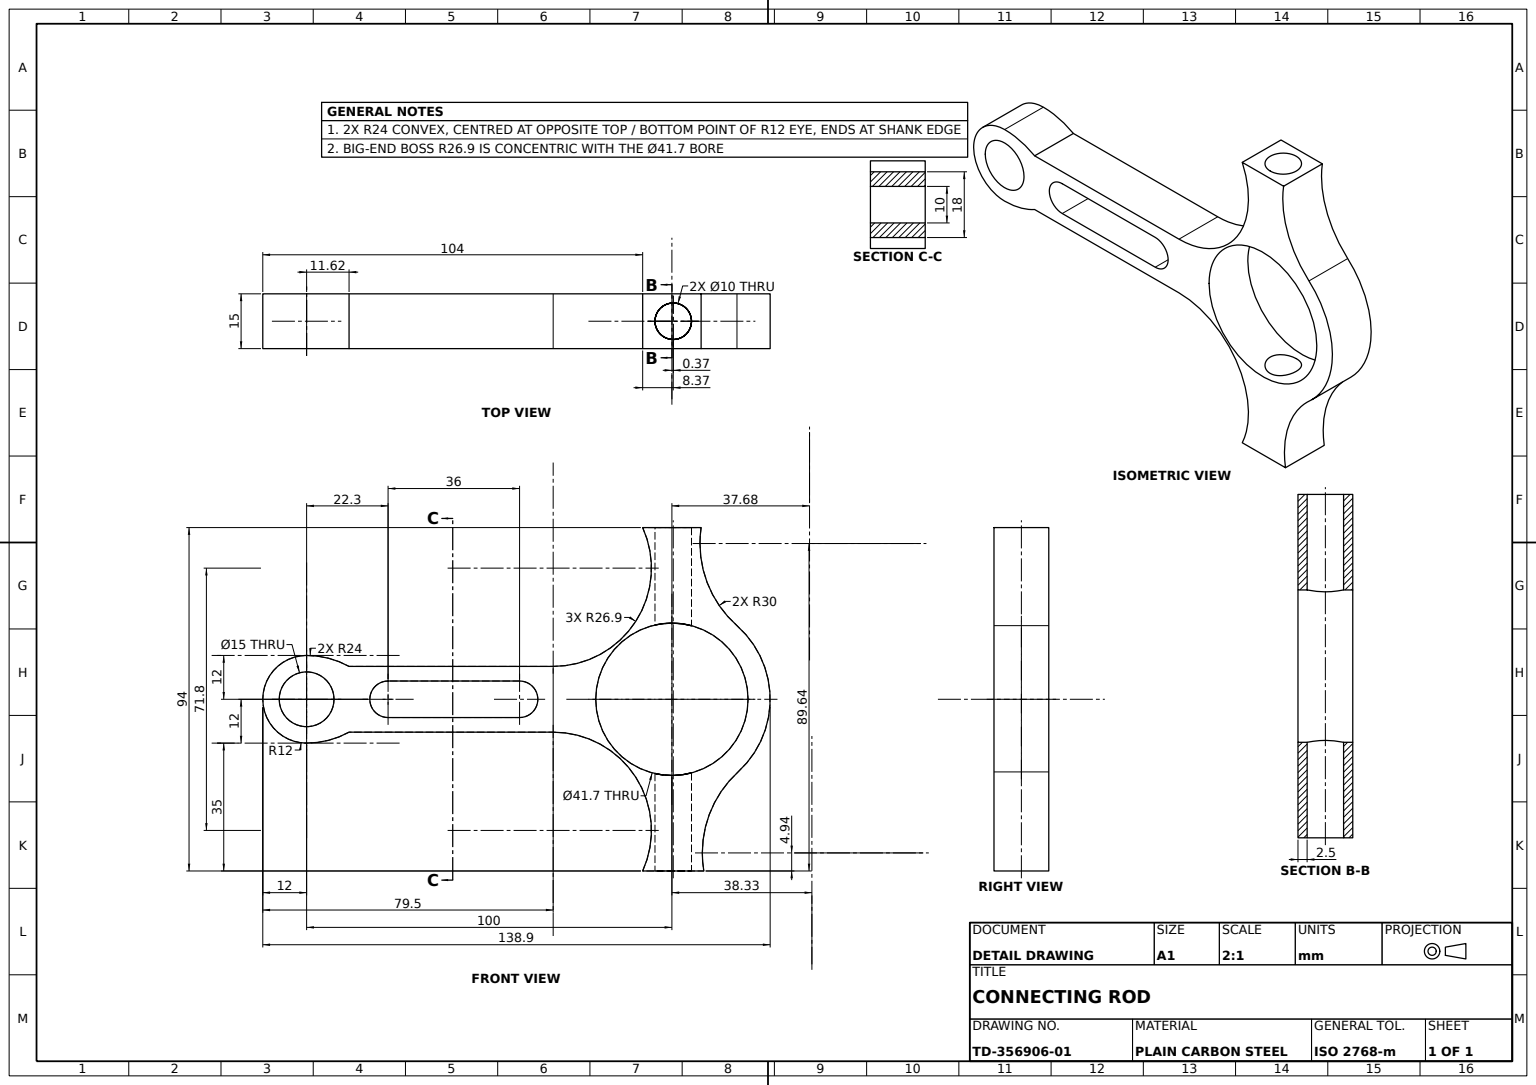
from build123d import *

# Parameters (mm, degrees)
LINK_PROFILE_SKETCH_R   = 7.5
LINK_PROFILE_SKETCH_R_2 = 20.85
LINK_BODY_15MM_DEPTH    = 15
BOLT_HOLE_SKETCH_R      = 5
BOLT_HOLE_10_DEPTH      = 159.633571478


with BuildPart() as part:
    # Link Profile Sketch → Link Body 15mm (new body)
    with BuildSketch(Plane.XY):
        with BuildLine():
            Line((100, 47), (92, 47))
            ThreePointArc((92, 47), (90.104459839, 21.32227727), (67.496938967, 9))
            Line((67.496938967, 9), (11.618950039, 9))
            ThreePointArc((11.618950039, 9), (6, 11.237900077), (0, 12))
            ThreePointArc((0, 12), (-12, 0), (0, -12))
            ThreePointArc((0, -12), (6, -11.237900077), (11.618950039, -9))
            Line((11.618950039, -9), (67.496938967, -9))
            ThreePointArc((67.496938967, -9), (90.104459839, -21.32227727), (92, -47))
            Line((92, -47), (100, -47))
            Line((100, -47), (108.73655718, -47))
            ThreePointArc((108.73655718, -47), (109.975380436, -32.246626192), (118.119137608, -19.882325124))
            ThreePointArc((118.119137608, -19.882325124), (126.899218543, 0.205040931), (117.813941305, 20.156227206))
            ThreePointArc((117.813941305, 20.156227206), (109.504751294, 32.334280207), (108, 47))
            Line((108, 47), (100, 47))
        make_face()
        Circle(LINK_PROFILE_SKETCH_R, mode=Mode.SUBTRACT)
        with Locations((100, 0)):
            Circle(LINK_PROFILE_SKETCH_R_2, mode=Mode.SUBTRACT)
        with BuildLine():
            Line((22.3, -5), (58.3, -5))
            ThreePointArc((58.3, -5), (63.3, 0), (58.3, 5))
            Line((58.3, 5), (22.3, 5))
            ThreePointArc((22.3, 5), (17.3, 0), (22.3, -5))
        make_face(mode=Mode.SUBTRACT)
    extrude(amount=LINK_BODY_15MM_DEPTH)

    # Bolt Hole Sketch → Bolt Hole Ø10 (cut, through all)
    with BuildSketch(Plane.XZ.offset(47)):
        with Locations(Location((100.36827859, 7.5, 0), (0, 0, 270))):
            Circle(BOLT_HOLE_SKETCH_R)
    extrude(amount=-BOLT_HOLE_10_DEPTH, mode=Mode.SUBTRACT)


solid = part.part
